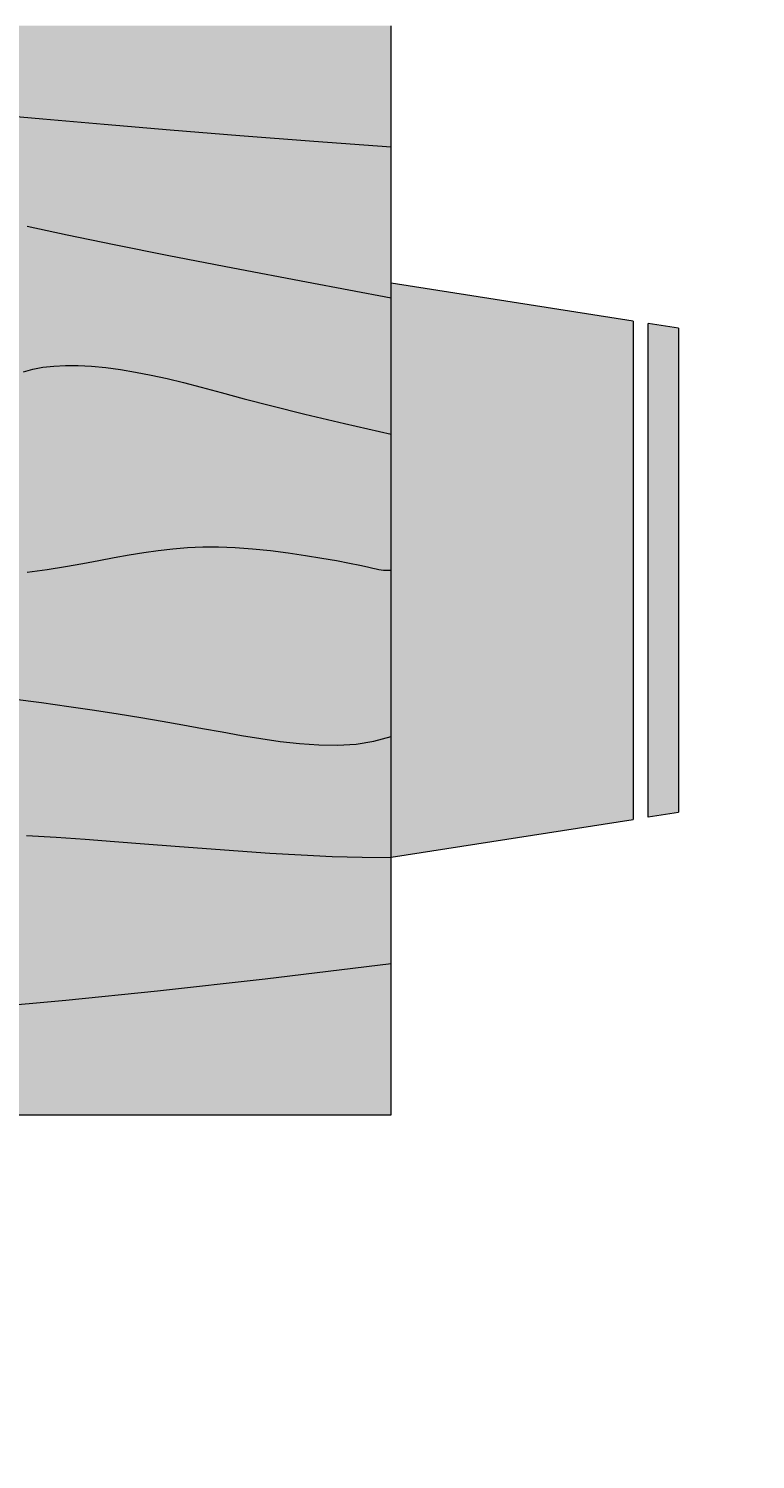
# Model space of a CAD drawing. Units: inches. Extents: x 2549 to 3108, y 1683 to 2362.
# Tile 13 of 30: x 2749 to 2762, y 2016 to 2041. Entities that reach past the tile are written whole.
import ezdxf

# ---------------------------------------------------------------- set-up
doc = ezdxf.new("R2010")
doc.units = ezdxf.units.IN
for name, color, linetype, lineweight in [('A-ANNO-DIMS', 2, 'Continuous', 18), ('A-FURN', 8, 'Continuous', 18), ('A-FURN-PATT', 9, 'Continuous', 13)]:
    doc.layers.add(name, color=color, linetype=linetype, lineweight=lineweight)
doc.layers.add('C-PKNG-VEHI-PATT', color=251, linetype='Continuous', lineweight=13, true_color=0x636466)
doc.layers.add('C-PVMT-PATT', color=9, linetype='Continuous', lineweight=13, true_color=0xc7c8ca)
doc.styles.get("Standard").update_dxf_attribs({"font": 'arial.ttf'})
doc.dimstyles.get("Standard").update_dxf_attribs({"dimtxt": 0.18, "dimasz": 0.18, "dimexe": 0.18, "dimexo": 0.0625, "dimgap": 0.09, "dimtad": 0, "dimtih": 1, "dimtoh": 1, "dimdec": 4, "dimzin": 0, "dimdsep": 46, "dimtxsty": 'Standard', "dimcen": 0.09, "dimadec": 0, "dimazin": 0, "dimtfac": 1, "dimtdec": 4, "dimtofl": 0, "dimtmove": 0, "dimatfit": 3, "dimfxl": 1, "dimtolj": 1, "dimtzin": 0, "dimarcsym": 0})

# ---------------------------------------------------------------- blocks, each defined once
blk = doc.blocks.new('Dining Set - 36 x 72 in.')
for p, q in [((36, -18), (36, 18)), ((44.0006, 8.23428), (35.9976, 9.48474)), ((44, 8.23041), (44, -8.23915)), ((44.5, -8.15843), (44.5, 8.15338)), ((45.5, 8), (44.5005, 8.15617)), ((45.5, 8), (45.5, -8)), ((44.4997, -8.15631), (45.5, -8)), ((35.9976, -9.48476), (43.9993, -8.2345)), ((-36, -18), (36, -18))]:
    blk.add_line(p, q)
for points in [[(22.5879, 15.08984), (24.4721, 14.91715), (26.5052, 14.73958), (28.6809, 14.5581), (30.9929, 14.3737), (33.4347, 14.18733), (36, 14)], [(23.959, 11.37304), (25.2786, 11.08618), (26.8282, 10.76562), (28.6414, 10.40405), (30.752, 9.99414), (33.1936, 9.52856), (36, 9)], [(23.8358, 6.55957), (24.142, 6.64323), (24.4735, 6.70735), (24.8334, 6.75), (25.2235, 6.76969), (25.642, 6.76692), (26.0858, 6.74267), (26.5521, 6.69791), (27.0379, 6.63362), (27.5404, 6.55078), (28.0565, 6.45036), (28.5834, 6.33333), (29.1242, 6.19987), (29.7071, 6.04687), (30.3661, 5.87044), (31.1354, 5.66666), (32.0493, 5.43164), (33.142, 5.16146), (34.4475, 4.85221), (36, 4.5)], [(23.9549, -0.06836), (24.6146, 0.02083), (25.2235, 0.11784), (25.7904, 0.21875), (26.3241, 0.31966), (26.8334, 0.41666), (27.3265, 0.50618), (27.8099, 0.58593), (28.2894, 0.65397), (28.7709, 0.70833), (29.2601, 0.74707), (29.763, 0.76823), (30.2855, 0.76985), (30.8334, 0.75), (31.4088, 0.70784), (31.9994, 0.64713), (32.589, 0.57275), (33.1615, 0.48958), (33.7008, 0.4025), (34.1908, 0.3164), (34.6153, 0.23616), (34.9584, 0.16666), (35.2099, 0.11165), (35.3848, 0.07031), (35.504, 0.04069), (35.5886, 0.02083), (35.6594, 0.00879), (35.7377, 0.0026), (35.8442, 0.00032), (36, 0)], [(23.4727, -4.25391), (24.4289, -4.37549), (25.3334, -4.5), (26.1785, -4.62492), (26.9694, -4.74935), (27.7145, -4.87281), (28.4219, -4.99479), (29.1, -5.11483), (29.7572, -5.23242), (30.4016, -5.34709), (31.0417, -5.45834), (31.6837, -5.56437), (32.3262, -5.65821), (32.9658, -5.73153), (33.599, -5.77604), (34.2224, -5.78345), (34.8327, -5.74545), (35.4264, -5.65373), (36, -5.5)], [(23.9271, -8.76563), (24.9081, -8.82707), (25.8763, -8.89388), (26.8465, -8.96558), (27.8334, -9.04167), (28.8474, -9.12118), (29.8828, -9.20117), (30.93, -9.27824), (31.9792, -9.34896), (33.0205, -9.40991), (34.0443, -9.45768), (35.0407, -9.48885), (36, -9.5)], [(-4.9224, -14.11833), (-3.0905, -14.16016), (-1.3709, -14.20785), (0.2448, -14.26042), (1.7647, -14.3169), (3.1973, -14.3763), (4.5507, -14.43767), (5.8333, -14.5), (7.0554, -14.5621), (8.235, -14.62175), (9.3922, -14.67652), (10.5469, -14.72396), (11.7192, -14.76164), (12.929, -14.78711), (14.1965, -14.79794), (15.5417, -14.79167), (16.9933, -14.76424), (18.6152, -14.70508), (20.4804, -14.60197), (22.6615, -14.44271), (25.2312, -14.21509), (28.2624, -13.9069), (31.8277, -13.50594), (36, -13)]]:
    blk.add_lwpolyline(points)
blk = doc.blocks.new('*D43')
at = {"layer": 'A-ANNO-DIMS', "color": 0, "lineweight": -2, "transparency": 16777216}
for p, q in [((2734.643, 2080.461), (2734.643, 1683.444)), ((2806.643, 2080.461), (2806.643, 1683.444)), ((2734.823, 1683.624), (2770.425, 1683.624)), ((2806.463, 1683.624), (2770.86, 1683.624))]:
    blk.add_line(p, q, dxfattribs=at)
at = {"layer": 'A-ANNO-DIMS', "color": 0, "transparency": 16777216}
for points in [[(2734.823, 1683.654), (2734.823, 1683.594), (2734.643, 1683.624)], [(2806.463, 1683.654), (2806.463, 1683.594), (2806.643, 1683.624)]]:
    blk.add_solid(points, dxfattribs=at)
at = {"layer": 'Defpoints', "color": 0, "transparency": 16777216}
for p in [(2734.643, 2080.524), (2806.643, 2080.524), (2806.643, 1683.624)]:
    blk.add_point(p, dxfattribs=at)
at = {"layer": 'A-ANNO-DIMS', "color": 0, "transparency": 16777216, "insert": (2770.643, 1683.624), "char_height": 0.18, "attachment_point": 5}
blk.add_mtext('\\A1;72', dxfattribs=at)
blk = doc.blocks.new('*D44')
at = {"layer": 'A-ANNO-DIMS', "color": 0, "lineweight": -2, "transparency": 16777216}
for p, q in [((2662.643, 2040.993), (2662.643, 1683.444)), ((2806.643, 2016.129), (2806.643, 1683.444)), ((2662.823, 1683.624), (2734.363, 1683.624)), ((2806.463, 1683.624), (2734.923, 1683.624))]:
    blk.add_line(p, q, dxfattribs=at)
at = {"layer": 'A-ANNO-DIMS', "color": 0, "transparency": 16777216}
for points in [[(2662.823, 1683.654), (2662.823, 1683.594), (2662.643, 1683.624)], [(2806.463, 1683.654), (2806.463, 1683.594), (2806.643, 1683.624)]]:
    blk.add_solid(points, dxfattribs=at)
at = {"layer": 'Defpoints', "color": 0, "transparency": 16777216}
for p in [(2662.643, 2041.056), (2806.643, 2016.191), (2806.643, 1683.624)]:
    blk.add_point(p, dxfattribs=at)
at = {"layer": 'A-ANNO-DIMS', "color": 0, "transparency": 16777216, "insert": (2734.643, 1683.624), "char_height": 0.18, "attachment_point": 5}
blk.add_mtext('\\A1;144', dxfattribs=at)
blk = doc.blocks.new('*D59')
at = {"layer": 'A-ANNO-DIMS', "color": 0, "lineweight": -2, "transparency": 16777216}
for p, q in [((2680.978, 1761.586), (2680.978, 2362.323)), ((2681.158, 2362.143), (2733.112, 2362.143)), ((2785.978, 2362.143), (2734.023, 2362.143)), ((2786.158, 1761.586), (2786.158, 2362.323))]:
    blk.add_line(p, q, dxfattribs=at)
at = {"layer": 'A-ANNO-DIMS', "color": 0, "transparency": 16777216}
for points in [[(2681.158, 2362.173), (2681.158, 2362.113), (2680.978, 2362.143)], [(2785.978, 2362.173), (2785.978, 2362.113), (2786.158, 2362.143)]]:
    blk.add_solid(points, dxfattribs=at)
at = {"layer": 'Defpoints', "color": 0, "transparency": 16777216}
for p in [(2786.158, 2362.143), (2680.978, 1761.524), (2786.158, 1761.524)]:
    blk.add_point(p, dxfattribs=at)
at = {"layer": 'A-ANNO-DIMS', "color": 0, "transparency": 16777216, "insert": (2733.568, 2362.143), "char_height": 0.18, "attachment_point": 5}
blk.add_mtext('\\A1;105.18', dxfattribs=at)

msp = doc.modelspace()

# ---------------------------------------------------------------- hatches: boundary and pattern name
at = {"layer": 'A-FURN-PATT'}
h = msp.add_hatch(color=256, dxfattribs=at)
h.dxf.hatch_style = 1
h.paths.add_polyline_path([(2732.9458, 2045.4744), (2724.0631, 2045.4744), (2723.389, 2041.1594), (2733.6201, 2041.1594)])
h.paths.add_polyline_path([(2748.0481, 2045.4744), (2739.1654, 2045.4744), (2738.4912, 2041.1594), (2748.7223, 2041.1594)])
h.paths.add_polyline_path([(2747.9217, 2046.2834), (2739.2918, 2046.2834), (2739.2075, 2045.7441), (2748.006, 2045.7441)])
h.paths.add_polyline_path([(2732.8194, 2046.2834), (2724.1896, 2046.2834), (2724.1053, 2045.7441), (2732.9037, 2045.7441)])
h.paths.add_polyline_path([(2759.7877, 2035.8922), (2755.4728, 2036.5664), (2755.4728, 2026.3353), (2759.7877, 2027.0095)])
h.paths.add_polyline_path([(2760.5968, 2035.7658), (2760.0574, 2035.8501), (2760.0574, 2027.0516), (2760.5968, 2027.1359)])
h.paths.add_polyline_path([(2716.6384, 2036.5664), (2712.3235, 2035.8922), (2712.3235, 2027.0095), (2716.6384, 2026.3353)])
h.paths.add_polyline_path([(2733.6201, 2021.7423), (2723.389, 2021.7423), (2724.0631, 2017.4273), (2732.9458, 2017.4273)])
h.paths.add_polyline_path([(2748.7223, 2021.7423), (2738.4912, 2021.7423), (2739.1654, 2017.4273), (2748.0481, 2017.4273)])
h.paths.add_polyline_path([(2748.006, 2017.1576), (2739.2075, 2017.1576), (2739.2918, 2016.6183), (2747.9217, 2016.6183)])
h.paths.add_polyline_path([(2732.9037, 2017.1576), (2724.1053, 2017.1576), (2724.1896, 2016.6183), (2732.8194, 2016.6183)])
h.paths.add_polyline_path([(2712.0538, 2035.85), (2711.5145, 2035.7658), (2711.5145, 2027.1359), (2712.0538, 2027.0516)])
h = msp.add_hatch(color=256, dxfattribs=at)
h.dxf.hatch_style = 1
h.paths.add_polyline_path([(2744.8667, 2037.254), (2744.7754, 2037.3839), (2744.7125, 2037.4849), (2744.6595, 2037.5854), (2744.5963, 2037.7375), (2744.5695, 2037.9287), (2744.6003, 2038.0617), (2744.6406, 2038.148), (2744.7014, 2038.2298), (2744.7817, 2038.3053), (2744.8799, 2038.3724), (2744.9945, 2038.4289), (2745.1238, 2038.4728), (2745.2663, 2038.5019), (2745.4204, 2038.5142), (2745.5844, 2038.5076), (2745.7585, 2038.4805), (2745.9486, 2038.4342), (2746.1624, 2038.3705), (2746.4075, 2038.2913), (2746.6917, 2038.1983), (2747.0224, 2038.0936), (2747.4074, 2037.9788), (2747.8543, 2037.8558), (2748.3724, 2037.7256), (2748.9783, 2037.5851), (2749.69, 2037.4304), (2750.5258, 2037.2575), (2751.5038, 2037.0624), (2752.6422, 2036.8414), (2753.9591, 2036.5902), (2755.4728, 2036.3051), (2755.4728, 2039.002), (2754.0892, 2039.103), (2752.7721, 2039.2035), (2751.5251, 2039.303), (2750.3516, 2039.4009), (2749.255, 2039.4967), (2748.2388, 2039.5898), (2747.3063, 2039.6798), (2746.4609, 2039.7661), (2745.7045, 2039.8482), (2745.0321, 2039.9255), (2744.4371, 2039.9976), (2743.9129, 2040.0639), (2743.4531, 2040.1238), (2743.0509, 2040.1769), (2742.6998, 2040.2227), (2742.3932, 2040.2605), (2742.1251, 2040.29), (2741.8917, 2040.3111), (2741.69, 2040.3237), (2741.5167, 2040.3279), (2741.3687, 2040.3237), (2741.2428, 2040.3111), (2741.1359, 2040.29), (2741.0448, 2040.2605), (2740.9668, 2040.2227), (2740.9015, 2040.1776), (2740.8488, 2040.1262), (2740.8088, 2040.0695), (2740.7814, 2040.0085), (2740.7667, 2039.9445), (2740.7646, 2039.8783), (2740.7751, 2039.811), (2740.7978, 2039.7435), (2740.8306, 2039.6755), (2740.8707, 2039.6064), (2740.9155, 2039.5357), (2740.996, 2039.4111), (2741.0771, 2039.2637), (2741.1346, 2039.0945), (2741.1499, 2038.9139), (2741.1092, 2038.7391), (2741.0289, 2038.6239), (2740.9549, 2038.5525), (2740.8586, 2038.4895), (2740.733, 2038.4359), (2740.5693, 2038.3929), (2740.3593, 2038.3615), (2740.0946, 2038.3427), (2739.7666, 2038.3376), (2739.367, 2038.3473), (2738.8873, 2038.3727), (2738.3203, 2038.4145), (2737.6635, 2038.471), (2736.9156, 2038.5402), (2736.0753, 2038.6199), (2735.1412, 2038.7081), (2734.112, 2038.8025), (2732.9864, 2038.9012), (2731.7632, 2039.002), (2730.4376, 2039.1026), (2728.9922, 2039.2), (2727.4062, 2039.2911), (2725.6588, 2039.3728), (2723.7291, 2039.4418), (2721.5964, 2039.495), (2719.2397, 2039.5292), (2716.6384, 2039.5413), (2716.6384, 2036.8445), (2720.4266, 2036.9215), (2723.5572, 2036.9548), (2726.1183, 2036.9512), (2728.1983, 2036.9175), (2729.8853, 2036.8608), (2731.2677, 2036.7876), (2732.4336, 2036.705), (2733.4711, 2036.6198), (2734.4538, 2036.5375), (2735.3951, 2036.4589), (2736.2938, 2036.3835), (2737.1484, 2036.3108), (2737.9578, 2036.2401), (2738.7205, 2036.171), (2739.4353, 2036.103), (2740.1009, 2036.0355), (2740.7163, 2035.9683), (2741.2828, 2035.9027), (2741.8019, 2035.8403), (2742.2752, 2035.7826), (2742.7042, 2035.7313), (2743.0906, 2035.6878), (2743.4358, 2035.6539), (2743.7416, 2035.6309), (2744.0097, 2035.6203), (2744.243, 2035.6218), (2744.4448, 2035.6349), (2744.6181, 2035.659), (2744.7661, 2035.6937), (2744.892, 2035.7384), (2744.9989, 2035.7926), (2745.09, 2035.8557), (2745.1679, 2035.9271), (2745.2326, 2036.006), (2745.2836, 2036.0911), (2745.3204, 2036.1815), (2745.3424, 2036.2762), (2745.3492, 2036.374), (2745.3401, 2036.4739), (2745.3148, 2036.5748), (2745.2731, 2036.676), (2745.2178, 2036.7771), (2745.152, 2036.8782), (2745.0788, 2036.9794), (2745.0013, 2037.0805)])
h.paths.add_polyline_path([(2755.4728, 2036.3051), (2753.9591, 2036.5902), (2752.6422, 2036.8414), (2751.5038, 2037.0624), (2750.5258, 2037.2575), (2749.69, 2037.4304), (2748.9783, 2037.5851), (2748.3724, 2037.7256), (2747.8543, 2037.8558), (2747.4074, 2037.9788), (2747.0224, 2038.0936), (2746.6917, 2038.1983), (2746.4075, 2038.2913), (2746.1624, 2038.3705), (2745.9486, 2038.4342), (2745.7585, 2038.4805), (2745.5844, 2038.5076), (2745.4204, 2038.5142), (2745.2663, 2038.5019), (2745.1238, 2038.4728), (2744.9945, 2038.4289), (2744.8799, 2038.3724), (2744.7817, 2038.3053), (2744.7014, 2038.2298), (2744.6406, 2038.148), (2744.6003, 2038.0617), (2744.5794, 2037.9717), (2744.5765, 2037.8786), (2744.59, 2037.7828), (2744.6182, 2037.6849), (2744.6595, 2037.5854), (2744.7125, 2037.4849), (2744.7754, 2037.3839), (2744.8465, 2037.2827), (2744.9229, 2037.1816), (2745.0013, 2037.0805), (2745.1278, 2036.9154), (2745.2178, 2036.7771), (2745.2731, 2036.676), (2745.3148, 2036.5748), (2745.3401, 2036.4739), (2745.3492, 2036.374), (2745.3424, 2036.2762), (2745.3204, 2036.1815), (2745.2836, 2036.0911), (2745.2326, 2036.006), (2745.1679, 2035.9271), (2745.09, 2035.8557), (2744.9989, 2035.7926), (2744.892, 2035.7384), (2744.7661, 2035.6937), (2744.6181, 2035.659), (2744.4448, 2035.6349), (2744.243, 2035.6218), (2744.0097, 2035.6203), (2743.7416, 2035.6309), (2743.4358, 2035.6539), (2743.0906, 2035.6878), (2742.7042, 2035.7313), (2742.2752, 2035.7826), (2741.8019, 2035.8403), (2741.2828, 2035.9027), (2740.7163, 2035.9683), (2740.1009, 2036.0355), (2739.4353, 2036.103), (2738.7205, 2036.171), (2737.9578, 2036.2401), (2737.1484, 2036.3108), (2736.2938, 2036.3835), (2735.3951, 2036.4589), (2734.4538, 2036.5375), (2733.4711, 2036.6198), (2732.4336, 2036.705), (2731.2677, 2036.7876), (2729.8853, 2036.8608), (2728.1983, 2036.9175), (2726.1183, 2036.9512), (2723.5572, 2036.9548), (2720.4266, 2036.9215), (2716.6384, 2036.8445), (2716.6384, 2034.4174), (2719.4886, 2034.3283), (2721.9949, 2034.2608), (2724.1925, 2034.2112), (2726.1167, 2034.1758), (2727.8028, 2034.1509), (2729.2861, 2034.1329), (2730.602, 2034.1181), (2731.7856, 2034.1027), (2732.8685, 2034.0839), (2733.8666, 2034.0613), (2734.7919, 2034.0356), (2735.6567, 2034.0072), (2736.473, 2033.9768), (2737.253, 2033.9447), (2738.0088, 2033.9116), (2738.7525, 2033.878), (2739.493, 2033.8445), (2740.2273, 2033.812), (2740.9489, 2033.7816), (2741.6515, 2033.7544), (2742.3289, 2033.7314), (2742.9747, 2033.7137), (2743.5825, 2033.7022), (2744.1461, 2033.6982), (2744.6607, 2033.7024), (2745.1272, 2033.7151), (2745.5485, 2033.7361), (2745.9272, 2033.7656), (2746.2658, 2033.8036), (2746.567, 2033.8499), (2746.8334, 2033.9047), (2747.0677, 2033.9679), (2747.2728, 2034.0393), (2747.4525, 2034.1175), (2747.6113, 2034.201), (2747.7531, 2034.2881), (2747.8824, 2034.3774), (2748.0032, 2034.4672), (2748.1197, 2034.556), (2748.2363, 2034.6421), (2748.3567, 2034.7241), (2748.4828, 2034.8008), (2748.6163, 2034.8712), (2748.7588, 2034.9343), (2748.9118, 2034.9889), (2749.077, 2035.034), (2749.2558, 2035.0686), (2749.4499, 2035.0916), (2749.6603, 2035.1022), (2749.8861, 2035.1007), (2750.1254, 2035.0876), (2750.3769, 2035.0635), (2750.639, 2035.0288), (2750.91, 2034.9841), (2751.1884, 2034.93), (2751.4725, 2034.8668), (2751.7642, 2034.7949), (2752.0786, 2034.7123), (2752.4341, 2034.6172), (2752.849, 2034.5073), (2753.3419, 2034.3805), (2753.9313, 2034.2348), (2754.6354, 2034.068), (2755.4728, 2033.878)])
h.paths.add_polyline_path([(2755.4728, 2033.878), (2754.6354, 2034.068), (2753.9313, 2034.2348), (2753.3419, 2034.3805), (2752.849, 2034.5073), (2752.4341, 2034.6172), (2752.0786, 2034.7123), (2751.7642, 2034.7949), (2751.4725, 2034.8668), (2751.1884, 2034.93), (2750.91, 2034.9841), (2750.639, 2035.0288), (2750.3769, 2035.0635), (2750.1254, 2035.0876), (2749.8861, 2035.1007), (2749.6603, 2035.1022), (2749.4499, 2035.0916), (2749.2558, 2035.0686), (2749.077, 2035.034), (2748.9118, 2034.9889), (2748.7588, 2034.9343), (2748.6163, 2034.8712), (2748.4828, 2034.8008), (2748.3567, 2034.7241), (2748.2363, 2034.6421), (2748.1197, 2034.556), (2748.0032, 2034.4672), (2747.8824, 2034.3774), (2747.7531, 2034.2881), (2747.6113, 2034.201), (2747.4525, 2034.1175), (2747.2728, 2034.0393), (2747.0677, 2033.9679), (2746.8334, 2033.9047), (2746.567, 2033.8499), (2746.2658, 2033.8036), (2745.9272, 2033.7656), (2745.5485, 2033.7361), (2745.1272, 2033.7151), (2744.6607, 2033.7024), (2744.1461, 2033.6982), (2743.5825, 2033.7022), (2742.9747, 2033.7137), (2742.3289, 2033.7314), (2741.6515, 2033.7544), (2740.9489, 2033.7816), (2740.2273, 2033.812), (2739.493, 2033.8445), (2738.7525, 2033.878), (2738.0088, 2033.9116), (2737.253, 2033.9447), (2736.473, 2033.9768), (2735.6567, 2034.0072), (2734.7919, 2034.0356), (2733.8666, 2034.0613), (2732.8685, 2034.0839), (2731.7856, 2034.1027), (2730.602, 2034.1181), (2729.2861, 2034.1329), (2727.8028, 2034.1509), (2726.1167, 2034.1758), (2724.1925, 2034.2112), (2721.9949, 2034.2608), (2719.4886, 2034.3283), (2716.6384, 2034.4174), (2716.6384, 2030.9115), (2719.4477, 2031.0954), (2722.0216, 2031.2447), (2724.3773, 2031.363), (2726.5324, 2031.4537), (2728.5042, 2031.5201), (2730.3101, 2031.5657), (2731.9674, 2031.5939), (2733.4936, 2031.6082), (2734.9046, 2031.6115), (2736.2109, 2031.6057), (2737.4211, 2031.592), (2738.5446, 2031.5716), (2739.59, 2031.5461), (2740.5665, 2031.5165), (2741.4829, 2031.4843), (2742.3482, 2031.4509), (2743.1698, 2031.4174), (2743.9488, 2031.3855), (2744.6845, 2031.3568), (2745.3766, 2031.3329), (2746.0244, 2031.3152), (2746.6274, 2031.3055), (2747.1851, 2031.3052), (2747.697, 2031.316), (2748.1634, 2031.3388), (2748.5882, 2031.3722), (2748.9761, 2031.414), (2749.3319, 2031.4621), (2749.6603, 2031.5144), (2749.9661, 2031.5688), (2750.254, 2031.6233), (2750.5287, 2031.6756), (2750.7946, 2031.7239), (2751.0553, 2031.7669), (2751.314, 2031.8036), (2751.5737, 2031.8329), (2751.8375, 2031.8538), (2752.1088, 2031.8652), (2752.3906, 2031.8661), (2752.6861, 2031.8554), (2752.9965, 2031.8326), (2753.315, 2031.7999), (2753.633, 2031.7598), (2753.9418, 2031.7149), (2754.2327, 2031.6679), (2754.497, 2031.6215), (2754.7259, 2031.5782), (2754.911, 2031.5407), (2755.0467, 2031.5111), (2755.141, 2031.4888), (2755.2053, 2031.4728), (2755.2509, 2031.4621), (2755.2891, 2031.4556), (2755.3313, 2031.4523), (2755.3888, 2031.451), (2755.4728, 2031.4509)])
h.paths.add_polyline_path([(2743.9488, 2031.3855), (2743.1698, 2031.4174), (2742.3482, 2031.4509), (2741.4829, 2031.4843), (2740.5665, 2031.5165), (2739.59, 2031.5461), (2738.5446, 2031.5716), (2737.4211, 2031.592), (2736.2109, 2031.6057), (2734.9046, 2031.6115), (2733.4936, 2031.6082), (2731.9674, 2031.5939), (2730.3101, 2031.5657), (2728.5042, 2031.5201), (2726.5324, 2031.4537), (2724.3773, 2031.363), (2722.0216, 2031.2447), (2719.4477, 2031.0954), (2716.6384, 2030.9115), (2716.6384, 2027.945), (2721.3933, 2028.046), (2725.223, 2028.1465), (2728.2515, 2028.246), (2730.603, 2028.3439), (2732.4013, 2028.4397), (2733.7707, 2028.5328), (2734.8351, 2028.6228), (2735.7185, 2028.7091), (2736.5253, 2028.7912), (2737.2808, 2028.8692), (2737.9904, 2028.9429), (2738.6597, 2029.0125), (2739.2943, 2029.0778), (2739.8997, 2029.1389), (2740.4813, 2029.1958), (2741.0448, 2029.2484), (2741.5952, 2029.2967), (2742.1361, 2029.3397), (2742.6708, 2029.3764), (2743.2022, 2029.4058), (2743.7337, 2029.4266), (2744.2683, 2029.4381), (2744.8093, 2029.4389), (2745.3597, 2029.4282), (2745.9213, 2029.4053), (2746.4897, 2029.3713), (2747.0592, 2029.3279), (2747.6239, 2029.2765), (2748.1781, 2029.2189), (2748.716, 2029.1564), (2749.2317, 2029.0909), (2749.7196, 2029.0237), (2750.1754, 2028.9563), (2750.602, 2028.8892), (2751.0039, 2028.8226), (2751.3854, 2028.7568), (2751.7512, 2028.6921), (2752.1057, 2028.6287), (2752.4532, 2028.5668), (2752.7985, 2028.5068), (2753.1447, 2028.4496), (2753.4913, 2028.399), (2753.8363, 2028.3595), (2754.1778, 2028.3355), (2754.514, 2028.3315), (2754.8432, 2028.352), (2755.1634, 2028.4014), (2755.4728, 2028.4843), (2755.4728, 2031.4509), (2755.3151, 2031.4512), (2755.2429, 2031.4634), (2755.141, 2031.4888), (2755.0467, 2031.5111), (2754.911, 2031.5407), (2754.7259, 2031.5782), (2754.497, 2031.6215), (2754.2327, 2031.6679), (2753.9418, 2031.7149), (2753.633, 2031.7598), (2753.315, 2031.7999), (2752.9965, 2031.8326), (2752.6861, 2031.8554), (2752.3906, 2031.8661), (2752.1088, 2031.8652), (2751.8375, 2031.8538), (2751.5737, 2031.8329), (2751.314, 2031.8036), (2751.0553, 2031.7669), (2750.7946, 2031.7239), (2750.5287, 2031.6756), (2750.254, 2031.6233), (2749.9661, 2031.5688), (2749.6603, 2031.5144), (2749.3319, 2031.4621), (2748.9761, 2031.414), (2748.5882, 2031.3722), (2748.1634, 2031.3388), (2747.697, 2031.316), (2747.1851, 2031.3052), (2746.6274, 2031.3055), (2746.0244, 2031.3152), (2745.3766, 2031.3329), (2744.6845, 2031.3568)])
h.paths.add_polyline_path([(2755.4728, 2028.4843), (2755.1634, 2028.4014), (2754.8432, 2028.352), (2754.514, 2028.3315), (2754.1778, 2028.3355), (2753.8363, 2028.3595), (2753.4913, 2028.399), (2753.1447, 2028.4496), (2752.7985, 2028.5068), (2752.4532, 2028.5668), (2752.1057, 2028.6287), (2751.7512, 2028.6921), (2751.3854, 2028.7568), (2751.0039, 2028.8226), (2750.602, 2028.8892), (2750.1754, 2028.9563), (2749.7196, 2029.0237), (2749.2317, 2029.0909), (2748.716, 2029.1564), (2748.1781, 2029.2189), (2747.6239, 2029.2765), (2747.0592, 2029.3279), (2746.4897, 2029.3713), (2745.9213, 2029.4053), (2745.3597, 2029.4282), (2744.8093, 2029.4389), (2744.2683, 2029.4381), (2743.7337, 2029.4266), (2743.2022, 2029.4058), (2742.6708, 2029.3764), (2742.1361, 2029.3397), (2741.5952, 2029.2967), (2741.0448, 2029.2484), (2740.4813, 2029.1958), (2739.8997, 2029.1389), (2739.2943, 2029.0778), (2738.6597, 2029.0125), (2737.9904, 2028.9429), (2737.2808, 2028.8692), (2736.5253, 2028.7912), (2735.7185, 2028.7091), (2734.8351, 2028.6228), (2733.7707, 2028.5328), (2732.4013, 2028.4397), (2730.603, 2028.3439), (2728.2515, 2028.246), (2725.223, 2028.1465), (2721.3933, 2028.046), (2716.6384, 2027.945), (2716.6384, 2023.63), (2719.8271, 2023.719), (2722.5536, 2023.7853), (2724.8739, 2023.8315), (2726.8443, 2023.8604), (2728.5207, 2023.8745), (2729.9593, 2023.8765), (2731.2162, 2023.8691), (2732.3475, 2023.8548), (2733.4006, 2023.8359), (2734.3887, 2023.8133), (2735.3162, 2023.7876), (2736.1877, 2023.7593), (2737.0074, 2023.7288), (2737.7801, 2023.6968), (2738.5101, 2023.6637), (2739.2019, 2023.63), (2739.8611, 2023.5965), (2740.4973, 2023.5644), (2741.1215, 2023.5348), (2741.7443, 2023.5092), (2742.3766, 2023.4889), (2743.0291, 2023.4752), (2743.7127, 2023.4693), (2744.4383, 2023.4727), (2745.2212, 2023.4875), (2746.096, 2023.5194), (2747.1021, 2023.575), (2748.2785, 2023.6609), (2749.6645, 2023.7837), (2751.2994, 2023.9499), (2753.2224, 2024.1662), (2755.4728, 2024.4391)])
h.paths.add_polyline_path([(2755.4728, 2026.3269), (2754.9554, 2026.3329), (2754.418, 2026.3497), (2753.8658, 2026.3755), (2753.3041, 2026.4083), (2752.7382, 2026.4465), (2752.1734, 2026.4881), (2751.6149, 2026.5312), (2751.068, 2026.5741), (2750.5357, 2026.6151), (2750.0124, 2026.6538), (2749.4902, 2026.6898), (2748.9611, 2026.723), (2748.4173, 2026.753), (2747.8508, 2026.7795), (2747.2537, 2026.8024), (2746.6182, 2026.8213), (2745.9367, 2026.8359), (2745.2024, 2026.8452), (2744.4091, 2026.8482), (2743.5505, 2026.8438), (2742.6204, 2026.8309), (2741.6122, 2026.8087), (2740.5198, 2026.7758), (2739.3368, 2026.7314), (2738.0388, 2026.6748), (2736.5297, 2026.6071), (2734.695, 2026.5299), (2732.4205, 2026.4449), (2729.5919, 2026.3535), (2726.0949, 2026.2573), (2721.8152, 2026.1581), (2716.6384, 2026.0572), (2716.6384, 2023.63), (2719.8271, 2023.719), (2722.5536, 2023.7853), (2724.8739, 2023.8315), (2726.8443, 2023.8604), (2728.5207, 2023.8745), (2729.9593, 2023.8765), (2731.2162, 2023.8691), (2732.3475, 2023.8548), (2733.4006, 2023.8359), (2734.3887, 2023.8133), (2735.3162, 2023.7876), (2736.1877, 2023.7593), (2737.0074, 2023.7288), (2737.7801, 2023.6968), (2738.5101, 2023.6637), (2739.2019, 2023.63), (2739.8611, 2023.5965), (2740.4973, 2023.5644), (2741.1215, 2023.5348), (2741.7443, 2023.5092), (2742.3766, 2023.4889), (2743.0291, 2023.4752), (2743.7127, 2023.4693), (2744.4383, 2023.4727), (2745.2212, 2023.4875), (2746.096, 2023.5194), (2747.1021, 2023.575), (2748.2785, 2023.6609), (2749.6645, 2023.7837), (2751.2994, 2023.9499), (2753.2224, 2024.1662), (2755.4728, 2024.4391)], flags=17)
h.paths.add_polyline_path([(2740.4973, 2023.5644), (2739.8611, 2023.5965), (2739.2019, 2023.63), (2738.5101, 2023.6637), (2737.7801, 2023.6968), (2737.0074, 2023.7288), (2736.1877, 2023.7593), (2735.3162, 2023.7876), (2734.3887, 2023.8133), (2733.4006, 2023.8359), (2732.3475, 2023.8548), (2731.2162, 2023.8691), (2729.9593, 2023.8765), (2728.5207, 2023.8745), (2726.8443, 2023.8604), (2724.8739, 2023.8315), (2722.5536, 2023.7853), (2719.8271, 2023.719), (2716.6384, 2023.63), (2716.6384, 2021.7423), (2755.4728, 2021.7423), (2755.4728, 2024.4391), (2753.2224, 2024.1662), (2751.2994, 2023.9499), (2749.6645, 2023.7837), (2748.2785, 2023.6609), (2747.1021, 2023.575), (2746.096, 2023.5194), (2745.2212, 2023.4875), (2744.4383, 2023.4727), (2743.7127, 2023.4693), (2743.0291, 2023.4752), (2742.3766, 2023.4889), (2741.7443, 2023.5092), (2741.1215, 2023.5348)])
h.paths.add_polyline_path([(2741.1359, 2040.29), (2741.2428, 2040.3111), (2741.3687, 2040.3237), (2741.5167, 2040.3279), (2741.69, 2040.3237), (2741.8917, 2040.3111), (2742.1251, 2040.29), (2742.3932, 2040.2605), (2742.6998, 2040.2227), (2743.0509, 2040.1769), (2743.4531, 2040.1238), (2743.9129, 2040.0639), (2744.4371, 2039.9976), (2745.0321, 2039.9255), (2745.7045, 2039.8482), (2746.4609, 2039.7661), (2747.3063, 2039.6798), (2748.2388, 2039.5898), (2749.255, 2039.4967), (2750.3516, 2039.4009), (2751.5251, 2039.303), (2752.7721, 2039.2035), (2754.0892, 2039.103), (2755.4728, 2039.002), (2755.4728, 2041.1594), (2716.6384, 2041.1594), (2716.6384, 2039.5413), (2719.2397, 2039.5292), (2721.5964, 2039.495), (2723.7291, 2039.4418), (2725.6588, 2039.3728), (2727.4062, 2039.2911), (2728.9922, 2039.2), (2730.4376, 2039.1026), (2731.7632, 2039.002), (2732.9864, 2038.9012), (2734.112, 2038.8025), (2735.1412, 2038.7081), (2736.0753, 2038.6199), (2736.9156, 2038.5402), (2737.6635, 2038.471), (2738.3203, 2038.4145), (2738.8873, 2038.3727), (2739.367, 2038.3473), (2739.7666, 2038.3376), (2740.0946, 2038.3427), (2740.3593, 2038.3615), (2740.5693, 2038.3929), (2740.733, 2038.4359), (2740.8586, 2038.4895), (2740.9549, 2038.5525), (2741.0289, 2038.6239), (2741.0834, 2038.7021), (2741.12, 2038.7856), (2741.1403, 2038.8728), (2741.1458, 2038.962), (2741.1382, 2039.0518), (2741.1189, 2039.1406), (2741.0897, 2039.2267), (2741.0522, 2039.309), (2741.0089, 2039.3875), (2740.9625, 2039.4629), (2740.8772, 2039.5951), (2740.8072, 2039.7159), (2740.7635, 2039.8453), (2740.7677, 2039.9782), (2740.8229, 2040.1009), (2740.9289, 2040.2044), (2741.0448, 2040.2605)])
h = msp.add_hatch(color=256, dxfattribs=at)
h.dxf.hatch_style = 1
h.paths.add_polyline_path([(2755.4728, 2026.3269), (2754.9554, 2026.3329), (2754.418, 2026.3497), (2753.8658, 2026.3755), (2753.3041, 2026.4083), (2752.7382, 2026.4465), (2752.1734, 2026.4881), (2751.6149, 2026.5312), (2751.068, 2026.5741), (2750.5357, 2026.6151), (2750.0124, 2026.6538), (2749.4902, 2026.6898), (2748.9611, 2026.723), (2748.4173, 2026.753), (2747.8508, 2026.7795), (2747.2537, 2026.8024), (2746.6182, 2026.8213), (2745.9367, 2026.8359), (2745.2024, 2026.8452), (2744.4091, 2026.8482), (2743.5505, 2026.8438), (2742.6204, 2026.8309), (2741.6122, 2026.8087), (2740.5198, 2026.7758), (2739.3368, 2026.7314), (2738.0388, 2026.6748), (2736.5297, 2026.6071), (2734.695, 2026.5299), (2732.4205, 2026.4449), (2729.5919, 2026.3535), (2726.0949, 2026.2573), (2721.8152, 2026.1581), (2716.6384, 2026.0572), (2716.6384, 2023.63), (2719.8271, 2023.719), (2722.5536, 2023.7853), (2724.8739, 2023.8315), (2726.8443, 2023.8604), (2728.5207, 2023.8745), (2729.9593, 2023.8765), (2731.2162, 2023.8691), (2732.3475, 2023.8548), (2733.4006, 2023.8359), (2734.3887, 2023.8133), (2735.3162, 2023.7876), (2736.1877, 2023.7593), (2737.0074, 2023.7288), (2737.7801, 2023.6968), (2738.5101, 2023.6637), (2739.2019, 2023.63), (2739.8611, 2023.5965), (2740.4973, 2023.5644), (2741.1215, 2023.5348), (2741.7443, 2023.5092), (2742.3766, 2023.4889), (2743.0291, 2023.4752), (2743.7127, 2023.4693), (2744.4383, 2023.4727), (2745.2212, 2023.4875), (2746.096, 2023.5194), (2747.1021, 2023.575), (2748.2785, 2023.6609), (2749.6645, 2023.7837), (2751.2994, 2023.9499), (2753.2224, 2024.1662), (2755.4728, 2024.4391)])
at = {"layer": 'C-PKNG-VEHI-PATT'}
h = msp.add_hatch(color=256, dxfattribs=at)
h.dxf.hatch_style = 1
edge = h.paths.add_edge_path()
edge.add_ellipse((2935.7258, 1791.964), major_axis=(-50.66, 0), ratio=0.8423039, start_angle=248.16505, end_angle=265.72258)
edge.add_line((2938.911, 1834.5507), (2925.8653, 1834.5507))
edge.add_ellipse((2929.0505, 1791.964), major_axis=(50.66, 0), ratio=0.8423039, start_angle=94.27742, end_angle=111.83495)
edge.add_line((2912.8508, 1832.3947), (2914.2044, 1822.2495))
edge.add_ellipse((2930.6538, 1783.1023), major_axis=(-49.3014, 0), ratio=0.8423039, start_angle=-85.12993, end_angle=-67.20809, ccw=False)
edge.add_line((2927.1247, 1824.5225), (2937.6516, 1824.5225))
edge.add_ellipse((2934.1225, 1783.1023), major_axis=(49.3014, 0), ratio=0.8423039, start_angle=67.20809, end_angle=85.12993, ccw=False)
edge.add_line((2950.5719, 1822.2495), (2951.9255, 1832.3947))
edge = h.paths.add_edge_path()
edge.add_ellipse((2903.4793, 1857.3351), major_axis=(-34.7979, 0), ratio=0.8423039, start_angle=180, end_angle=209.43857)
edge.add_ellipse((2961.297, 1857.3351), major_axis=(34.7979, 0), ratio=0.8423039, start_angle=150.56143, end_angle=180)
edge.add_line((2926.4991, 1857.3351), (2926.4991, 1843.7609))
edge.add_ellipse((2924.1251, 1844.3143), major_axis=(-0.2209, 3.9278), ratio=0.6038336, start_angle=89.00201, end_angle=253.65741, ccw=False)
edge.add_line((2921.7512, 1844.2222), (2921.7512, 1853.3975))
edge.add_line((2921.7512, 1853.3975), (2925.269, 1855.8484))
edge.add_ellipse((2925.4782, 1855.4931), major_axis=(0.4584, 0), ratio=0.8423039, start_angle=90, end_angle=134.48021, ccw=False)
edge.add_line((2925.4782, 1855.8792), (2926.4991, 1855.8792))
edge.add_line((2926.4991, 1855.8792), (2926.4991, 1857.3351))
edge.add_ellipse((2961.297, 1857.3351), major_axis=(34.7979, 0), ratio=0.8423039, start_angle=150.56143, end_angle=180, ccw=False)
edge.add_line((2932.3882, 1873.6501), (2932.3882, 1875.7801))
edge.add_ellipse((2932.3882, 1875.3939), major_axis=(0.4584, 0), ratio=0.8423039, start_angle=90, end_angle=127.93313)
edge.add_line((2932.1366, 1875.7167), (2928.5915, 1873.7564))
edge.add_ellipse((2899.9271, 2002.4692), major_axis=(155.4756, 0), ratio=0.84230387, start_angle=-80.743434, end_angle=-77.445067, ccw=False)
edge.add_ellipse((2949.4402, 1715.2151), major_axis=(-189.1422, 0), ratio=0.84230387, start_angle=-79.790461, end_angle=-77.555373)
edge.add_ellipse((3300.3614, 1852.5642), major_axis=(-386.1662, 0), ratio=0.84230387, start_angle=-2.863715, end_angle=2.198541)
edge.add_ellipse((2929.0505, 1792.5159), major_axis=(-55.6192, 0), ratio=0.8423039, start_angle=-85.91759, end_angle=-72.28005, ccw=False)
edge.add_line((2925.7129, 1839.2798), (2939.0634, 1839.2798))
edge.add_ellipse((2935.7258, 1792.5159), major_axis=(55.6192, 0), ratio=0.8423039, start_angle=72.28005, end_angle=85.91759, ccw=False)
edge.add_ellipse((2564.4149, 1852.5642), major_axis=(-386.1662, 0), ratio=0.84230387, start_angle=177.801459, end_angle=182.863715)
edge.add_ellipse((2915.3361, 1715.2151), major_axis=(189.1422, 0), ratio=0.84230387, start_angle=77.555373, end_angle=79.790461)
edge.add_ellipse((2964.8492, 2002.4692), major_axis=(-155.4756, 0), ratio=0.84230387, start_angle=77.445067, end_angle=80.743434, ccw=False)
edge.add_line((2936.1848, 1873.7564), (2932.6397, 1875.7167))
edge.add_ellipse((2932.3882, 1875.3939), major_axis=(0.4584, 0), ratio=0.8423039, start_angle=52.06687, end_angle=90)
edge.add_line((2932.3882, 1875.7801), (2932.3882, 1873.6501))
edge.add_ellipse((2903.4793, 1857.3351), major_axis=(-34.7979, 0), ratio=0.8423039, start_angle=180, end_angle=209.43857, ccw=False)
edge.add_line((2938.2772, 1857.3351), (2938.2772, 1855.8792))
edge.add_line((2938.2772, 1855.8792), (2939.4059, 1855.8792))
edge.add_ellipse((2939.2981, 1855.4931), major_axis=(-0.4584, 0), ratio=0.8423039, start_angle=225.51979, end_angle=270, ccw=False)
edge.add_line((2939.5903, 1855.7906), (2943.0251, 1853.3975))
edge.add_line((2943.0251, 1853.3975), (2943.0251, 1844.2222))
edge.add_ellipse((2940.6512, 1844.3143), major_axis=(0.2209, 3.9278), ratio=0.6038336, start_angle=106.34259, end_angle=270.99799, ccw=False)
edge.add_line((2938.2772, 1843.7609), (2938.2772, 1857.3351))
edge = h.paths.add_edge_path()
edge.add_ellipse((2932.3882, 1865.1973), major_axis=(91.081, 0), ratio=0.8423039, start_angle=256.401865, end_angle=283.598135, ccw=False)
edge.add_line((2914.2044, 1790.0239), (2914.2044, 1778.3622))
edge.add_ellipse((2932.3882, 1853.5356), major_axis=(91.081, 0), ratio=0.8423039, start_angle=256.401865, end_angle=283.598135)
edge.add_line((2950.5719, 1778.3622), (2950.5719, 1790.0239))
edge = h.paths.add_edge_path()
edge.add_ellipse((2948.7383, 1772.3145), major_axis=(1.8336, 0), ratio=0.8423039, start_angle=0, end_angle=90)
edge.add_line((2948.7383, 1773.859), (2916.038, 1773.859))
edge.add_ellipse((2916.038, 1772.3145), major_axis=(1.8336, 0), ratio=0.8423039, start_angle=90, end_angle=180)
edge.add_line((2914.2044, 1772.3145), (2914.2044, 1760.2558))
edge.add_line((2914.2044, 1760.2558), (2950.5719, 1760.2558))
edge.add_line((2950.5719, 1760.2558), (2950.5719, 1772.3145))
h.paths.add_polyline_path([(2748.8496, 2101.6383), (2798.148, 2101.6383), (2798.148, 2111.4248), (2748.8496, 2111.4248)], flags=9)
h.paths.add_polyline_path([(2685.2081, 2101.489), (2719.3253, 2101.489), (2719.3253, 2111.2819), (2685.2081, 2111.2819)], flags=9)
h.paths.add_polyline_path([(2814.6852, 1907.1328), (2847.8384, 1907.1328), (2847.8384, 1916.9258), (2814.6852, 1916.9258)], flags=9)
h.paths.add_polyline_path([(2814.3906, 1835.5864), (2848.0172, 1835.5864), (2848.0172, 1845.3794), (2814.3906, 1845.3794)], flags=9)
h.paths.add_polyline_path([(2800.5245, 1759.1674), (2853.7435, 1759.1674), (2853.7435, 1768.954), (2800.5245, 1768.954)], flags=9)
h.paths.add_polyline_path([(2972.4611, 1807.3305), (3015.3943, 1807.3305), (3015.3943, 1817.117), (2972.4611, 1817.117)], flags=9)
h.paths.add_polyline_path([(2902.3327, 1888.6731), (2937.9131, 1888.6731), (2937.9131, 1898.4661), (2902.3327, 1898.4661)], flags=9)
h.paths.add_polyline_path([(2712.1779, 1878.9039), (2754.1257, 1878.9039), (2754.1257, 1888.6904), (2712.1779, 1888.6904)], flags=9)
h.paths.add_polyline_path([(2614.0056, 2012.812), (2650.0251, 2012.812), (2650.0251, 2022.4371), (2614.0056, 2022.4371)], flags=9)
h.paths.add_polyline_path([(2713.3129, 2003.1645), (2747.4237, 2003.1645), (2747.4237, 2012.951), (2713.3129, 2012.951)], flags=9)
h.paths.add_polyline_path([(2950.1379, 2001.6934), (2982.2992, 2001.6934), (2982.2992, 2011.48), (2950.1379, 2011.48)], flags=9)
h.paths.add_polyline_path([(2940.864, 2238.5537), (2997.5066, 2238.5537), (2997.5066, 2248.3466), (2940.864, 2248.3466)], flags=9)
h.paths.add_polyline_path([(2821.5457, 2202.8348), (2855.663, 2202.8348), (2855.663, 2212.6278), (2821.5457, 2212.6278)], flags=9)
h.paths.add_polyline_path([(2661.8026, 2238.6249), (2718.4451, 2238.6249), (2718.4451, 2248.4179), (2661.8026, 2248.4179)], flags=9)
at = {"layer": 'C-PVMT-PATT'}
h = msp.add_hatch(color=256, dxfattribs=at)
h.dxf.hatch_style = 1
h.paths.add_polyline_path([(3067.6427, 2305.5237), (2605.6427, 2305.5237), (2605.6427, 2074.5237), (2629.6427, 2074.5237), (2629.6427, 2281.5237), (3043.6427, 2281.5237), (3043.6427, 1885.5237), (3043.6427, 1872.8745), (3031.1672, 1872.8745), (3031.1672, 1862.5731), (2995.8054, 1862.5731), (2995.8054, 1872.8745), (2983.1752, 1872.8745), (2983.1752, 1885.5237), (2881.6427, 1885.5237), (2881.6427, 1795.5237), (2751.0977, 1795.5237), (2751.0977, 1761.5237), (2786.1577, 1761.5237), (2786.1577, 1723.5237), (2881.84, 1723.5237), (2881.84, 1714.5237), (3067.6427, 1714.5237), (3067.6427, 1723.5237)])
edge = h.paths.add_edge_path(flags=16)
edge.add_ellipse((2949.4402, 1710.9683), major_axis=(-194.1014, 0), ratio=0.84230387, start_angle=-77.874034, end_angle=-76.219471, ccw=False)
edge.add_ellipse((2949.4402, 1715.2151), major_axis=(-189.1422, 0), ratio=0.84230387, start_angle=-79.790461, end_angle=-77.555373, ccw=False)
edge.add_ellipse((2899.9271, 2002.4692), major_axis=(155.4756, 0), ratio=0.84230387, start_angle=-80.743434, end_angle=-77.445067)
edge.add_line((2928.5915, 1873.7564), (2932.3882, 1875.8558))
edge.add_line((2932.3882, 1875.8558), (2936.1848, 1873.7564))
edge.add_ellipse((2964.8492, 2002.4692), major_axis=(-155.4756, 0), ratio=0.84230387, start_angle=77.445067, end_angle=80.743434)
edge.add_ellipse((2915.3361, 1715.2151), major_axis=(189.1422, 0), ratio=0.84230387, start_angle=77.555373, end_angle=79.790461, ccw=False)
edge.add_ellipse((2915.3361, 1710.9683), major_axis=(-194.1014, 0), ratio=0.84230387, start_angle=256.219471, end_angle=257.874034, ccw=False)
edge.add_ellipse((2628.2871, 1850.2612), major_axis=(-327.2532, 0), ratio=0.84230387, start_angle=182.17995, end_angle=183.650428, ccw=False)
edge.add_ellipse((2955.5637, 1861.9334), major_axis=(-0.9168, 0), ratio=0.8423039, start_angle=180, end_angle=270, ccw=False)
edge.add_line((2956.4805, 1862.3857), (2956.4805, 1846.4866))
edge.add_ellipse((2955.5637, 1846.939), major_axis=(-0.9168, 0), ratio=0.8423039, start_angle=90, end_angle=180, ccw=False)
edge.add_ellipse((-3607.0606, 1835.832), major_axis=(-6562.6242, 0), ratio=0.84230387, start_angle=179.61613322, end_angle=180.09022909, ccw=False)
edge.add_ellipse((2955.5637, 1791.0926), major_axis=(0.9168, 0), ratio=0.8423039, start_angle=0, end_angle=90, ccw=False)
edge.add_line((2956.4805, 1791.545), (2956.4805, 1775.6459))
edge.add_ellipse((2955.5637, 1776.0982), major_axis=(0.9168, 0), ratio=0.8423039, start_angle=270, end_angle=360, ccw=False)
edge.add_ellipse((-3607.0606, 1835.832), major_axis=(-6562.6242, 0), ratio=0.84230387, start_angle=179.3813568, end_angle=179.47172853, ccw=False)
edge.add_ellipse((2954.5907, 1763.8768), major_axis=(-1.3752, 0), ratio=0.8423039, start_angle=179.37176, end_angle=248.46476, ccw=False)
edge.add_ellipse((-3607.519, 1835.832), major_axis=(-6564.0409, 0), ratio=0.842303863, start_angle=179.35344594, end_angle=179.37176282, ccw=False)
edge.add_ellipse((2952.6829, 1761.8002), major_axis=(3.2503, 0), ratio=0.8423039, start_angle=-90, end_angle=-0.64655, ccw=False)
edge.add_line((2952.6829, 1759.0625), (2912.0934, 1759.0625))
edge.add_ellipse((2912.0934, 1761.8002), major_axis=(3.2503, 0), ratio=0.8423039, start_angle=180.64655, end_angle=270, ccw=False)
edge.add_ellipse((9472.2953, 1835.832), major_axis=(-6564.0409, 0), ratio=0.842303871, start_angle=0.62823722, end_angle=0.6465541, ccw=False)
edge.add_ellipse((2910.1856, 1763.8768), major_axis=(1.3752, 0), ratio=0.8423039, start_angle=111.53524, end_angle=180.62824, ccw=False)
edge.add_ellipse((9471.8369, 1835.832), major_axis=(-6562.6242, 0), ratio=0.84230387, start_angle=0.52827147, end_angle=0.6465541, ccw=False)
edge.add_ellipse((2909.2126, 1776.0982), major_axis=(-0.9168, 0), ratio=0.8423039, start_angle=0, end_angle=90, ccw=False)
edge.add_line((2908.2958, 1775.6459), (2908.2958, 1791.545))
edge.add_ellipse((2909.2126, 1791.0926), major_axis=(-0.9168, 0), ratio=0.8423039, start_angle=-90, end_angle=0, ccw=False)
edge.add_ellipse((9471.8369, 1835.832), major_axis=(-6562.6242, 0), ratio=0.84230387, start_angle=-0.09022909, end_angle=0.38386678, ccw=False)
edge.add_ellipse((2909.2126, 1846.939), major_axis=(-0.9168, 0), ratio=0.8423039, start_angle=0, end_angle=90, ccw=False)
edge.add_line((2908.2958, 1846.4866), (2908.2958, 1862.3857))
edge.add_ellipse((2909.2126, 1861.9334), major_axis=(0.9168, 0), ratio=0.8423039, start_angle=90, end_angle=180, ccw=False)
edge.add_ellipse((3236.4892, 1850.2612), major_axis=(327.2532, 0), ratio=0.84230387, start_angle=176.349572, end_angle=177.82005, ccw=False)
edge = h.paths.add_edge_path(flags=0)
edge.add_ellipse((2903.4793, 1857.3351), major_axis=(-34.7979, 0), ratio=0.8423039, start_angle=180, end_angle=209.43857, ccw=False)
edge.add_line((2938.2772, 1857.3351), (2938.2772, 1855.8792))
edge.add_line((2938.2772, 1855.8792), (2939.4631, 1855.8792))
edge.add_line((2939.4631, 1855.8792), (2943.0251, 1853.3975))
edge.add_line((2943.0251, 1853.3975), (2943.0251, 1844.2222))
edge.add_ellipse((2940.6512, 1844.3143), major_axis=(0.2209, 3.9278), ratio=0.6038336, start_angle=106.34259, end_angle=270.99799, ccw=False)
edge.add_line((2938.2772, 1843.7609), (2938.2772, 1857.3351))
edge.add_ellipse((2903.4793, 1857.3351), major_axis=(-34.7979, 0), ratio=0.8423039, start_angle=180, end_angle=209.43857)
edge.add_ellipse((2961.297, 1857.3351), major_axis=(34.7979, 0), ratio=0.8423039, start_angle=150.56143, end_angle=180)
edge.add_line((2926.4991, 1857.3351), (2926.4991, 1843.7609))
edge.add_ellipse((2924.1251, 1844.3143), major_axis=(-0.2209, 3.9278), ratio=0.6038336, start_angle=89.00201, end_angle=253.65741, ccw=False)
edge.add_line((2921.7512, 1844.2222), (2921.7512, 1853.3975))
edge.add_line((2921.7512, 1853.3975), (2925.3132, 1855.8792))
edge.add_line((2925.3132, 1855.8792), (2926.4991, 1855.8792))
edge.add_line((2926.4991, 1855.8792), (2926.4991, 1857.3351))
edge.add_ellipse((2961.297, 1857.3351), major_axis=(34.7979, 0), ratio=0.8423039, start_angle=150.56143, end_angle=180, ccw=False)
edge = h.paths.add_edge_path(flags=0)
edge.add_ellipse((2929.0505, 1791.964), major_axis=(50.66, 0), ratio=0.8423039, start_angle=94.27742, end_angle=111.83495, ccw=False)
edge.add_line((2925.8653, 1834.5507), (2938.911, 1834.5507))
edge.add_ellipse((2935.7258, 1791.964), major_axis=(-50.66, 0), ratio=0.8423039, start_angle=248.16505, end_angle=265.72258, ccw=False)
edge.add_line((2951.9255, 1832.3947), (2950.5719, 1822.2495))
edge.add_ellipse((2934.1225, 1783.1023), major_axis=(49.3014, 0), ratio=0.8423039, start_angle=67.20809, end_angle=85.12993)
edge.add_line((2937.6516, 1824.5225), (2927.1247, 1824.5225))
edge.add_ellipse((2930.6538, 1783.1023), major_axis=(-49.3014, 0), ratio=0.8423039, start_angle=-85.12993, end_angle=-67.20809)
edge.add_line((2914.2044, 1822.2495), (2912.8508, 1832.3947))
edge = h.paths.add_edge_path(flags=0)
edge.add_line((2910.1338, 1829.4651), (2912.6432, 1821.2711))
edge.add_ellipse((5203.7787, 1816.4367), major_axis=(-2291.1426, 0), ratio=0.84230387, start_angle=-0.1208974, end_angle=0.3640763)
edge.add_line((2912.7012, 1801.8782), (2910.3305, 1792.5698))
edge.add_ellipse((9471.8369, 1835.832), major_axis=(-6561.7074, 0), ratio=0.84230387, start_angle=0.05559431, end_angle=0.37776419, ccw=False)
edge = h.paths.add_edge_path(flags=0)
edge.add_ellipse((-3607.0606, 1835.832), major_axis=(6561.7074, 0), ratio=0.84230387, start_angle=-0.37776419, end_angle=-0.05559431, ccw=False)
edge.add_line((2954.4458, 1792.5698), (2952.0751, 1801.8782))
edge.add_ellipse((660.9976, 1816.4367), major_axis=(2291.1426, 0), ratio=0.84230387, start_angle=-0.3640763, end_angle=0.1208974)
edge.add_line((2952.1331, 1821.2711), (2954.6425, 1829.4651))
edge = h.paths.add_edge_path(flags=0)
edge.add_ellipse((2932.3882, 1865.1973), major_axis=(91.081, 0), ratio=0.8423039, start_angle=256.401865, end_angle=283.598135)
edge.add_line((2950.5719, 1790.0239), (2950.5719, 1778.3622))
edge.add_ellipse((2932.3882, 1853.5356), major_axis=(91.081, 0), ratio=0.8423039, start_angle=256.401865, end_angle=283.598135, ccw=False)
edge.add_line((2914.2044, 1778.3622), (2914.2044, 1790.0239))
edge = h.paths.add_edge_path(flags=0)
edge.add_line((2916.038, 1773.859), (2948.7383, 1773.859))
edge.add_ellipse((2948.7383, 1772.3145), major_axis=(1.8336, 0), ratio=0.8423039, start_angle=0, end_angle=90, ccw=False)
edge.add_line((2950.5719, 1772.3145), (2950.5719, 1760.2558))
edge.add_line((2950.5719, 1760.2558), (2914.2044, 1760.2558))
edge.add_line((2914.2044, 1760.2558), (2914.2044, 1772.3145))
edge.add_ellipse((2916.038, 1772.3145), major_axis=(1.8336, 0), ratio=0.8423039, start_angle=90, end_angle=180, ccw=False)
h.paths.add_polyline_path([(2629.6427, 1978.5237), (2605.6427, 1978.5237), (2605.6427, 1723.5237), (2629.6427, 1723.5237), (2629.6427, 1795.5237)], flags=17)
h.paths.add_polyline_path([(2800.5245, 1759.1674), (2853.7435, 1759.1674), (2853.7435, 1768.954), (2800.5245, 1768.954)], flags=24)
h.paths.add_polyline_path([(2972.4611, 1807.3305), (3015.3943, 1807.3305), (3015.3943, 1817.117), (2972.4611, 1817.117)], flags=24)

# ---------------------------------------------------------------- block references
at = {"layer": 'A-FURN', "xscale": 0.5393661791637867, "yscale": 0.5393661791637867, "zscale": 0.5393661791637867}
msp.add_blockref('Dining Set - 36 x 72 in.', (2736.0556, 2031.4509), dxfattribs=at)

# ---------------------------------------------------------------- dimensions: what is measured, and where the dimension line sits
at = {"layer": 'A-ANNO-DIMS'}
for base, p1, p2, override, picture, middle in [((2786.1577, 2362.1425), (2680.9778, 1761.5237), (2786.1577, 1761.5237), {"dimdec": 2, "dimlfac": 1, "dimrnd": 0, "dimzin": 0, "dimdsep": 46, "dimlunit": 2}, '*D59', (2733.5678, 2362.1425)), ((2806.6427, 1683.6237), (2734.6427, 2080.5237), (2806.6427, 2080.5237), {"dimdec": 0, "dimlfac": 1, "dimrnd": 0, "dimzin": 0, "dimdsep": 46, "dimlunit": 2}, '*D43', (2770.6427, 1683.6237)), ((2806.6427, 1683.6237), (2662.6427, 2041.0557), (2806.6427, 2016.1911), {"dimdec": 0, "dimlfac": 1, "dimrnd": 0, "dimzin": 0, "dimdsep": 46, "dimlunit": 2}, '*D44', (2734.6427, 1683.6237))]:
    dim = msp.add_linear_dim(base=base, p1=p1, p2=p2, dimstyle='Standard', override=override, dxfattribs=at)
    dim.commit()
    dim.dimension.update_dxf_attribs({"geometry": picture, "text_midpoint": middle})

doc.saveas('drawing.dxf')
